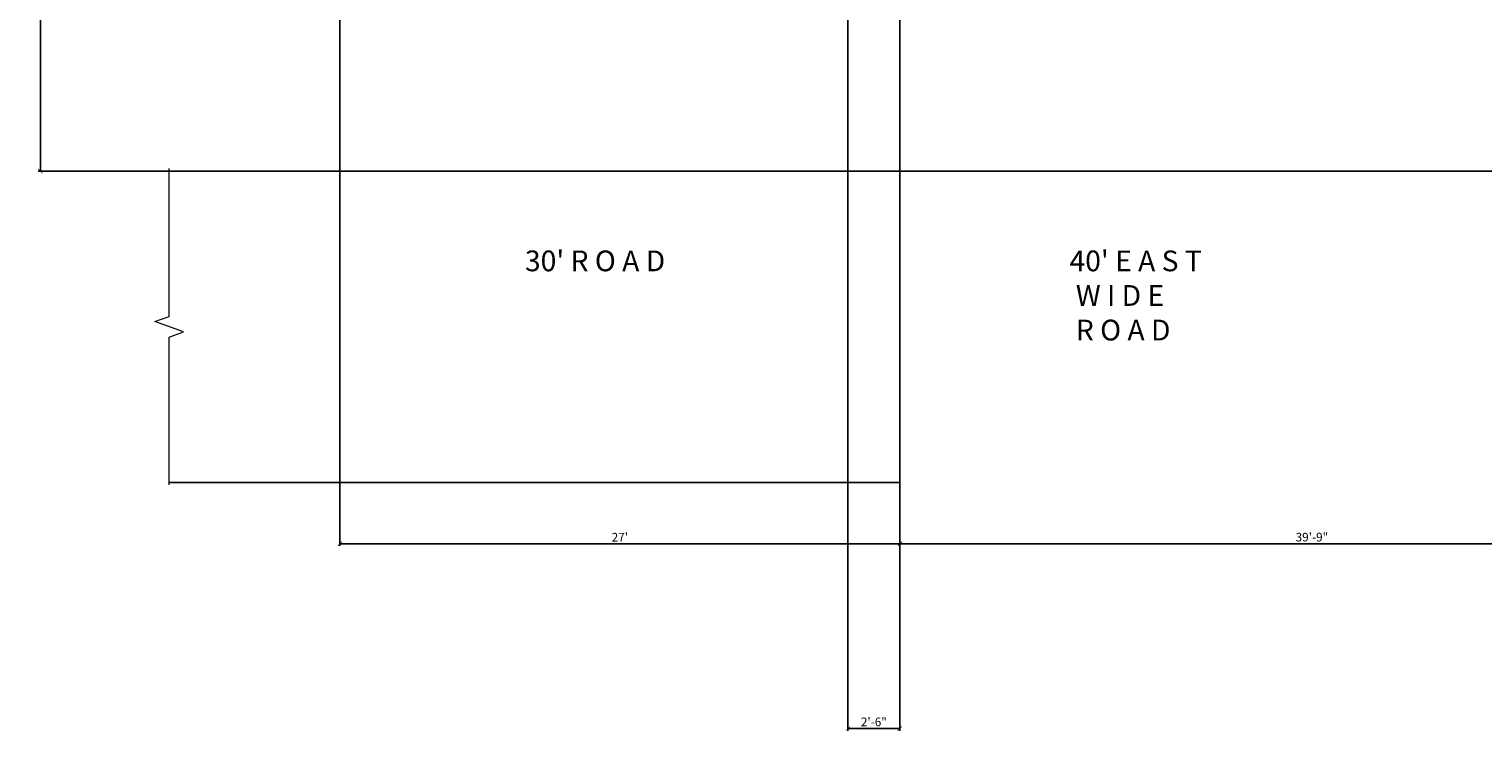
# Model space of a CAD drawing. Units: inches. Extents: x 3283068 to 3284536, y 3240756 to 3241803.
# Tile 1 of 19: x 3283068 to 3283910, y 3240759 to 3241165. Entities that reach past the tile are written whole.
import ezdxf

# ---------------------------------------------------------------- set-up
doc = ezdxf.new("R2010")
doc.units = ezdxf.units.IN
for name, color, linetype, lineweight in [('A-ANNO-DIMS', 2, 'Continuous', 18), ('C-ANNO-SYMB', 7, 'Continuous', 18), ('C-ANNO-TEXT', 7, 'Continuous', 18), ('C-PROP', 7, 'Continuous', 25), ('C-ROAD', 8, 'Continuous', 25)]:
    doc.layers.add(name, color=color, linetype=linetype, lineweight=lineweight)
doc.styles.get("Standard").update_dxf_attribs({"font": 'arial.ttf'})
doc.dimstyles.new('ISO-25', dxfattribs={"dimtxt": 5, "dimasz": 2.5, "dimexe": 1.25, "dimexo": 0.625, "dimtad": 1, "dimlunit": 4, "dimtxsty": 'Standard', "dimblk": 'ARCHTICK', "dimcen": 2.5, "dimadec": 0, "dimazin": 0, "dimtfac": 1, "dimtmove": 0, "dimatfit": 3, "dimfxl": 1, "dimarcsym": 0})

# ---------------------------------------------------------------- blocks, each defined once
blk = doc.blocks.new('_ArchTick')
at = {"color": 0, "linetype": 'ByBlock', "const_width": 0.15}
blk.add_lwpolyline([(-0.5, -0.5), (0.5, 0.5)], dxfattribs=at)
blk = doc.blocks.new('*D31')
at = {"layer": 'A-ANNO-DIMS', "color": 0, "lineweight": -2, "transparency": 16777216}
for p, q in [((3283248.09, 3241081.98), (3283248.09, 3240865.87)), ((3283572.09, 3240901.98), (3283572.09, 3240865.87)), ((3283248.09, 3240867.12), (3283572.09, 3240867.12))]:
    blk.add_line(p, q, dxfattribs=at)
at = {"layer": 'Defpoints', "color": 0, "transparency": 16777216}
for p in [(3283248.09, 3241082.6), (3283572.09, 3240902.6), (3283572.09, 3240867.12)]:
    blk.add_point(p, dxfattribs=at)
at = {"layer": 'A-ANNO-DIMS', "color": 0, "lineweight": -2, "transparency": 16777216, "xscale": 2.5, "yscale": 2.5, "zscale": 2.5, "rotation": 180}
blk.add_blockref('_ArchTick', (3283248.09, 3240867.12), dxfattribs=at)
at = {"layer": 'A-ANNO-DIMS', "color": 0, "lineweight": -2, "transparency": 16777216, "xscale": 2.5, "yscale": 2.5, "zscale": 2.5}
blk.add_blockref('_ArchTick', (3283572.09, 3240867.12), dxfattribs=at)
at = {"layer": 'A-ANNO-DIMS', "color": 0, "transparency": 16777216, "insert": (3283410.09, 3240870.26), "char_height": 5, "attachment_point": 5}
blk.add_mtext("27'", dxfattribs=at)
blk = doc.blocks.new('*D32')
at = {"layer": 'A-ANNO-DIMS', "color": 0, "lineweight": -2, "transparency": 16777216}
for p, q in [((3283572.09, 3240901.98), (3283572.09, 3240865.87)), ((3283572.09, 3240867.12), (3284049.09, 3240867.12)), ((3284049.09, 3240867.75), (3284049.09, 3240868.37))]:
    blk.add_line(p, q, dxfattribs=at)
at = {"layer": 'Defpoints', "color": 0, "transparency": 16777216}
for p in [(3283572.09, 3240902.6), (3284049.09, 3240867.12), (3284049.09, 3240867.12)]:
    blk.add_point(p, dxfattribs=at)
at = {"layer": 'A-ANNO-DIMS', "color": 0, "lineweight": -2, "transparency": 16777216, "xscale": 2.5, "yscale": 2.5, "zscale": 2.5, "rotation": 180}
blk.add_blockref('_ArchTick', (3283572.09, 3240867.12), dxfattribs=at)
at = {"layer": 'A-ANNO-DIMS', "color": 0, "lineweight": -2, "transparency": 16777216, "xscale": 2.5, "yscale": 2.5, "zscale": 2.5}
blk.add_blockref('_ArchTick', (3284049.09, 3240867.12), dxfattribs=at)
at = {"layer": 'A-ANNO-DIMS', "color": 0, "transparency": 16777216, "insert": (3283810.59, 3240870.3), "char_height": 5, "attachment_point": 5}
blk.add_mtext('39\'-9"', dxfattribs=at)
blk = doc.blocks.new('ROAD-BREAK')
blk.add_lwpolyline([(8.24, 0), (8.24, 85.5), (16.48, 88.5), (0, 94.5), (8.24, 97.5), (8.24, 183)])
blk = doc.blocks.new('*D61')
at = {"layer": 'A-ANNO-DIMS', "color": 0, "lineweight": -2, "transparency": 16777216}
for p, q in [((3283247.46, 3241730.6), (3283073.57, 3241730.6)), ((3283074.82, 3241082.6), (3283074.82, 3241730.6)), ((3283247.46, 3241082.6), (3283073.57, 3241082.6))]:
    blk.add_line(p, q, dxfattribs=at)
at = {"layer": 'Defpoints', "color": 0, "transparency": 16777216}
for p in [(3283074.82, 3241730.6), (3283248.09, 3241730.6), (3283248.09, 3241082.6)]:
    blk.add_point(p, dxfattribs=at)
at = {"layer": 'A-ANNO-DIMS', "color": 0, "lineweight": -2, "transparency": 16777216, "xscale": 2.5, "yscale": 2.5, "zscale": 2.5}
for p, rotation in [((3283074.82, 3241730.6), 90), ((3283074.82, 3241082.6), 270)]:
    blk.add_blockref('_ArchTick', p, dxfattribs=dict(at, rotation=rotation))
at = {"layer": 'A-ANNO-DIMS', "color": 0, "transparency": 16777216, "insert": (3283071.64, 3241406.6), "char_height": 5, "attachment_point": 5, "rotation": 90}
blk.add_mtext('54\'-0"', dxfattribs=at)
blk = doc.blocks.new('*D63')
at = {"layer": 'A-ANNO-DIMS', "color": 0, "lineweight": -2, "transparency": 16777216}
for p, q in [((3283248.09, 3241083.23), (3283248.09, 3241798.08)), ((3283248.09, 3241796.83), (3284328.09, 3241796.83)), ((3284328.09, 3241083.23), (3284328.09, 3241798.08))]:
    blk.add_line(p, q, dxfattribs=at)
at = {"layer": 'Defpoints', "color": 0, "transparency": 16777216}
for p in [(3284328.09, 3241796.83), (3283248.09, 3241082.6), (3284328.09, 3241082.6)]:
    blk.add_point(p, dxfattribs=at)
at = {"layer": 'A-ANNO-DIMS', "color": 0, "lineweight": -2, "transparency": 16777216, "xscale": 2.5, "yscale": 2.5, "zscale": 2.5, "rotation": 180}
blk.add_blockref('_ArchTick', (3283248.09, 3241796.83), dxfattribs=at)
at = {"layer": 'A-ANNO-DIMS', "color": 0, "lineweight": -2, "transparency": 16777216, "xscale": 2.5, "yscale": 2.5, "zscale": 2.5}
blk.add_blockref('_ArchTick', (3284328.09, 3241796.83), dxfattribs=at)
at = {"layer": 'A-ANNO-DIMS', "color": 0, "transparency": 16777216, "insert": (3283788.09, 3241800.01), "char_height": 5, "attachment_point": 5}
blk.add_mtext('90\'-0"', dxfattribs=at)
blk = doc.blocks.new('*D64')
at = {"layer": 'A-ANNO-DIMS', "color": 0, "lineweight": -2, "transparency": 16777216}
for p, q in [((3283542.09, 3241534.98), (3283542.09, 3240759.03)), ((3283572.09, 3241534.98), (3283572.09, 3240759.03)), ((3283542.09, 3240760.28), (3283572.09, 3240760.28))]:
    blk.add_line(p, q, dxfattribs=at)
at = {"layer": 'Defpoints', "color": 0, "transparency": 16777216}
for p in [(3283542.09, 3241535.6), (3283572.09, 3241535.6), (3283572.09, 3240760.28)]:
    blk.add_point(p, dxfattribs=at)
at = {"layer": 'A-ANNO-DIMS', "color": 0, "lineweight": -2, "transparency": 16777216, "xscale": 2.5, "yscale": 2.5, "zscale": 2.5, "rotation": 180}
blk.add_blockref('_ArchTick', (3283542.09, 3240760.28), dxfattribs=at)
at = {"layer": 'A-ANNO-DIMS', "color": 0, "lineweight": -2, "transparency": 16777216, "xscale": 2.5, "yscale": 2.5, "zscale": 2.5}
blk.add_blockref('_ArchTick', (3283572.09, 3240760.28), dxfattribs=at)
at = {"layer": 'A-ANNO-DIMS', "color": 0, "transparency": 16777216, "insert": (3283557.09, 3240763.46), "char_height": 5, "attachment_point": 5}
blk.add_mtext('2\'-6"', dxfattribs=at)

msp = doc.modelspace()

# ---------------------------------------------------------------- linework, layer by layer
at = {"layer": 'C-PROP'}
for p, q in [((3283248.089, 3241730.602), (3283248.089, 3241082.602)), ((3283248.089, 3241082.602), (3284328.089, 3241082.602))]:
    msp.add_line(p, q, dxfattribs=at)
at = {"layer": 'C-ROAD'}
for p, q in [((3283248.089, 3241082.602), (3283149.285, 3241082.602)), ((3283149.285, 3240902.602), (3283572.089, 3240902.602)), ((3283248.089, 3240902.602), (3283572.089, 3240902.602)), ((3283572.089, 3240902.602), (3283572.089, 3240826.506))]:
    msp.add_line(p, q, dxfattribs=at)

# ---------------------------------------------------------------- block references
at = {"layer": 'C-ANNO-SYMB'}
msp.add_blockref('ROAD-BREAK', (3283141.042, 3240901.102), dxfattribs=at)

# ---------------------------------------------------------------- texts
at = {"layer": 'C-ANNO-TEXT', "char_height": 12, "attachment_point": 1}
for s, width, insert in [("30' R O A D", 123.55873, (3283355.172, 3241036.697)), ("40' E A S T \\P W I D E\\P R O A D", 85.09051, (3283670.295, 3241036.697))]:
    msp.add_mtext_dynamic_manual_height_columns(s, width=width, gutter_width=12.5, heights=[0], dxfattribs=dict(at, insert=insert))

# ---------------------------------------------------------------- dimensions: what is measured, and where the dimension line sits
at = {"layer": 'A-ANNO-DIMS'}
for base, p1, p2, override, picture, middle in [((3284328.089, 3241796.827), (3283248.089, 3241082.602), (3284328.089, 3241082.602), {"dimdec": 1, "dimlfac": 1, "dimrnd": 0, "dimzin": 1, "dimdsep": 46, "dimlunit": 4, "dimfrac": 2}, '*D63', (3283788.089, 3241800.005)), ((3283572.089, 3240760.281), (3283542.089, 3241535.602), (3283572.089, 3241535.602), {"dimdec": 1, "dimlfac": 1, "dimrnd": 0, "dimzin": 1, "dimdsep": 46, "dimlunit": 4, "dimfrac": 2}, '*D64', (3283557.089, 3240763.459)), ((3283572.089, 3240867.124), (3283248.089, 3241082.602), (3283572.089, 3240902.602), {"dimclrd": 0, "dimclre": 0, "dimclrt": 0}, '*D31', (3283410.089, 3240870.259)), ((3284049.089, 3240867.124), (3283572.089, 3240902.602), (3284049.089, 3240867.124), {"dimclrd": 0, "dimclre": 0, "dimclrt": 0, "dimtmove": 1}, '*D32', (3283810.589, 3240870.304))]:
    dim = msp.add_linear_dim(base=base, p1=p1, p2=p2, dimstyle='ISO-25', override=override, dxfattribs=at)
    dim.commit()
    dim.dimension.update_dxf_attribs({"geometry": picture, "text_midpoint": middle})
dim = msp.add_linear_dim(base=(3283074.817, 3241730.602), p1=(3283248.089, 3241082.602), p2=(3283248.089, 3241730.602), angle=90, dimstyle='ISO-25', override={"dimdec": 1, "dimlfac": 1, "dimrnd": 0, "dimzin": 1, "dimdsep": 46, "dimlunit": 4, "dimfrac": 2}, dxfattribs=at)
dim.commit()
dim.dimension.update_dxf_attribs({"geometry": '*D61', "text_midpoint": (3283071.639, 3241406.602)})

doc.saveas('drawing.dxf')
